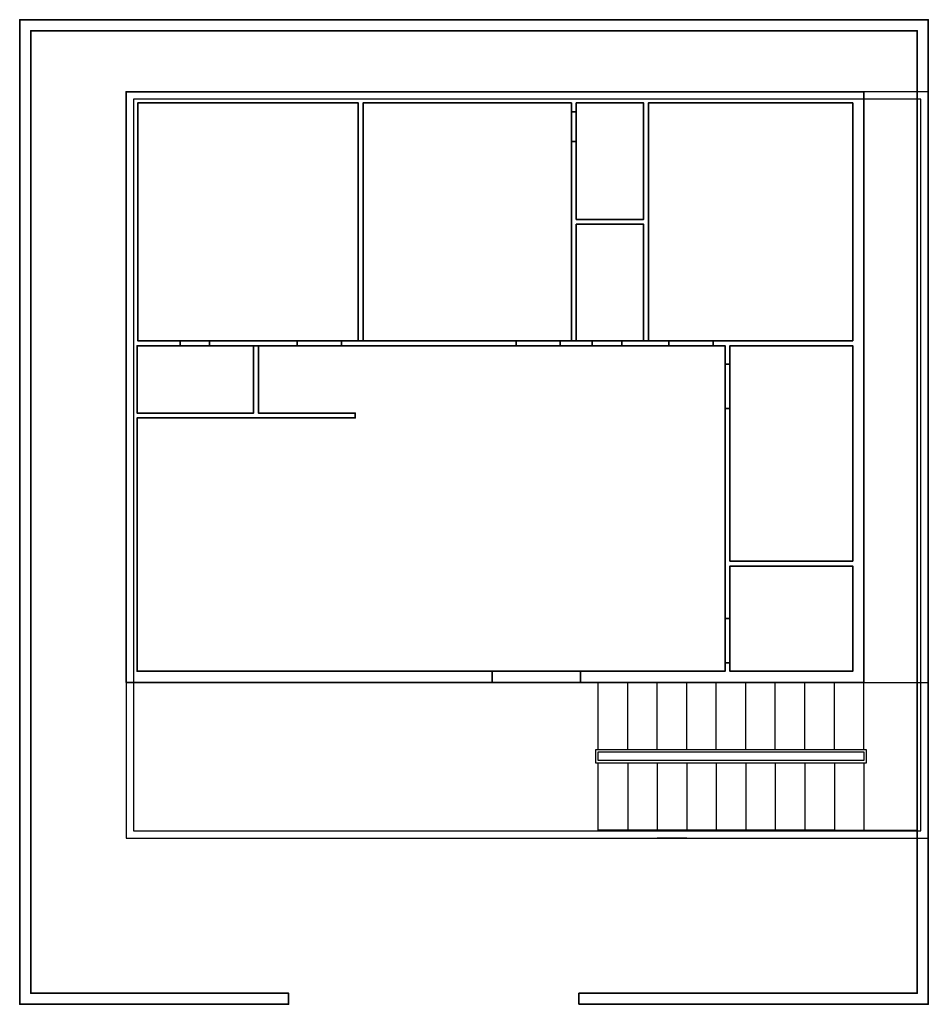
# Model space of a CAD drawing. Units: feet. Extents: x 3511 to 6270, y 2172 to 4127.
# Tile 3 of 4: x 5531 to 6270, y 2172 to 2972. Entities that reach past the tile are written whole.
import ezdxf

# ---------------------------------------------------------------- set-up
doc = ezdxf.new("R2010")
doc.units = ezdxf.units.FT
for name, color, linetype, lineweight in [('A-FLOR-OTLN', 3, 'Continuous', 25), ('A-FLOR-STRS', 4, 'Continuous', 25), ('A-WALL', 7, 'Continuous', 35), ('C-PROP', 1, 'Continuous', 35)]:
    doc.layers.add(name, color=color, linetype=linetype, lineweight=lineweight)

msp = doc.modelspace()

# ---------------------------------------------------------------- linework, layer by layer
at = {"layer": 'A-FLOR-OTLN', "elevation": 414}
for points in [[(5617.51, 2306.9), (6269.92, 2306.9), (6269.92, 2913.43), (5617.51, 2913.43)], [(5623.51, 2312.9), (6263.92, 2312.9), (6263.92, 2907.43), (5623.51, 2907.43)]]:
    msp.add_lwpolyline(points, close=True, dxfattribs=at)
at = {"layer": 'A-FLOR-STRS'}
for p, q in [((6001.51, 2379.01), (6001.51, 2433.43)), ((6025.51, 2379.01), (6025.51, 2433.43)), ((6049.51, 2379.01), (6049.51, 2433.43)), ((6073.51, 2379.01), (6073.51, 2433.43)), ((6097.51, 2379.01), (6097.51, 2433.43)), ((6121.51, 2379.01), (6121.51, 2433.43)), ((6145.51, 2379.01), (6145.51, 2433.43)), ((6169.51, 2379.01), (6169.51, 2433.43)), ((6193.51, 2379.01), (6193.51, 2433.43)), ((6260.92, 2433.43, 60), (6269.92, 2433.43, 60)), ((6269.92, 2306.9, 60), (6269.92, 2433.43, 60)), ((6217.51, 2367.86), (6217.51, 2313.43)), ((6217.51, 2313.43, 50.56), (6260.92, 2313.43, 50.56)), ((6049.51, 2306.9, 246), (6073.51, 2306.9, 246)), ((6073.51, 2306.9, 120), (6049.51, 2306.9, 120)), ((6260.92, 2306.9, 60), (6269.92, 2306.9, 60))]:
    msp.add_line(p, q, dxfattribs=at)
for points in [[(6217.51, 2379.01), (6217.51, 2433.43), (6260.92, 2433.43)], [(6025.51, 2367.86), (6025.51, 2313.43), (6013.51, 2313.43), (6001.51, 2313.43), (6001.51, 2367.86)], [(6049.51, 2367.86), (6049.51, 2313.43), (6037.51, 2313.43), (6025.51, 2313.43)], [(6073.51, 2367.86), (6073.51, 2313.43), (6061.51, 2313.43), (6049.51, 2313.43)], [(6097.51, 2367.86), (6097.51, 2313.43), (6085.51, 2313.43), (6073.51, 2313.43)], [(6121.51, 2367.86), (6121.51, 2313.43), (6109.51, 2313.43), (6097.51, 2313.43)], [(6145.51, 2367.86), (6145.51, 2313.43), (6133.51, 2313.43), (6121.51, 2313.43)], [(6169.51, 2367.86), (6169.51, 2313.43), (6157.51, 2313.43), (6145.51, 2313.43)], [(6193.51, 2367.86), (6193.51, 2313.43), (6181.51, 2313.43), (6169.51, 2313.43)], [(6193.51, 2313.43), (6205.51, 2313.43), (6217.51, 2313.43), (6260.92, 2313.43)]]:
    msp.add_lwpolyline(points, dxfattribs=at)
for points in [[(5999.51, 2379.01), (6219.51, 2379.01), (6219.51, 2367.86), (5999.51, 2367.86)], [(6217.51, 2369.86), (6001.51, 2369.86), (6001.51, 2377.01), (6217.51, 2377.01)]]:
    msp.add_lwpolyline(points, close=True, dxfattribs=at)
at = {"layer": 'A-WALL'}
msp.add_lwpolyline([(6108.6, 2528), (6108.6, 2485.38), (6104.6, 2485.38), (6104.6, 2656), (6108.6, 2656), (6108.6, 2532), (6208.51, 2532), (6208.51, 2707.06), (6108.6, 2707.06), (6108.6, 2692), (6104.6, 2692), (6104.6, 2707.06), (6094.92, 2707.06), (6094.92, 2711.06), (6208.51, 2711.06), (6208.51, 2904.43), (6042.38, 2904.43), (6042.38, 2711.06), (6058.92, 2711.06), (6058.92, 2707.06), (6020.61, 2707.06), (6020.61, 2711.06), (6038.38, 2711.06), (6038.38, 2805.75), (5983.67, 2805.75), (5983.67, 2711.06), (5996.61, 2711.06), (5996.61, 2707.06), (5970.67, 2707.06), (5970.67, 2711.06), (5979.67, 2711.06), (5979.67, 2873.18), (5983.67, 2873.18), (5983.67, 2809.75), (6038.38, 2809.75), (6038.38, 2904.43), (5983.67, 2904.43), (5983.67, 2897.18), (5979.67, 2897.18), (5979.67, 2904.43), (5810.34, 2904.43), (5810.34, 2711.06), (5934.67, 2711.06), (5934.67, 2707.06), (5792.78, 2707.06), (5792.78, 2711.06), (5806.34, 2711.06), (5806.34, 2904.43), (5627, 2904.43), (5627, 2711.06), (5661.53, 2711.06), (5661.53, 2707.06), (5626.51, 2707.06), (5626.51, 2652.36), (5626.51, 2652.36), (5721.2, 2652.36), (5721.2, 2707.07), (5685.53, 2707.07), (5685.53, 2711.07), (5756.78, 2711.07), (5756.78, 2707.07), (5725.2, 2707.07), (5725.2, 2652.36), (5803.95, 2652.36), (5803.95, 2648.36), (5626.51, 2648.36), (5626.51, 2442.43), (5915.15, 2442.43), (5915.15, 2433.43), (5617.51, 2433.43), (5617.51, 2913.43), (6217.51, 2913.43), (6217.51, 2433.43), (5987.15, 2433.43), (5987.15, 2442.43), (6104.6, 2442.43), (6104.6, 2449.38), (6108.6, 2449.38), (6108.6, 2442.43), (6208.51, 2442.43), (6208.51, 2528)], close=True, dxfattribs=at)
at = {"layer": 'A-WALL', "elevation": 120}
for points in [[(6217.51, 2433.43), (5617.51, 2433.43), (5617.51, 2913.43), (6217.51, 2913.43), (6217.51, 2433.43)], [(5806.34, 2711.06), (5806.34, 2904.43), (5627, 2904.43), (5627, 2711.06), (6208.51, 2711.06), (6208.51, 2904.43), (6042.38, 2904.43), (6042.38, 2711.06)], [(5979.67, 2904.43), (5810.34, 2904.43), (5810.34, 2711.06)], [(5979.67, 2711.06), (5979.67, 2904.43)], [(5983.67, 2904.43), (5983.67, 2809.75), (6038.38, 2809.75), (6038.38, 2904.43), (5983.67, 2904.43)], [(6038.38, 2711.06), (6038.38, 2805.75), (5983.67, 2805.75), (5983.67, 2711.06)], [(5725.2, 2707.07), (5725.2, 2652.36), (5803.95, 2652.36), (5803.95, 2648.36), (5626.51, 2648.36), (5626.51, 2442.43), (6104.6, 2442.43), (6104.6, 2707.06), (5626.51, 2707.06), (5626.51, 2652.36), (5626.51, 2652.36), (5721.2, 2652.36), (5721.2, 2707.07)], [(6108.6, 2707.06), (6108.6, 2532), (6208.51, 2532), (6208.51, 2707.06), (6108.6, 2707.06)], [(6108.6, 2442.43), (6208.51, 2442.43), (6208.51, 2528), (6108.6, 2528), (6108.6, 2442.43)]]:
    msp.add_lwpolyline(points, dxfattribs=at)
at = {"layer": 'A-WALL'}
msp.add_lwpolyline([(5725.2, 2648.36), (5725.2, 2648.36)], dxfattribs=at)
at = {"layer": 'C-PROP'}
msp.add_lwpolyline([(5985.75, 2171.8), (6269.92, 2171.8), (6269.92, 2972.04), (5531.06, 2972.04), (5531.06, 2171.8), (5749.68, 2171.8), (5749.68, 2180.8), (5540.06, 2180.8), (5540.06, 2963.04), (6260.92, 2963.04), (6260.92, 2180.8), (5985.75, 2180.8)], close=True, dxfattribs=at)

doc.saveas('drawing.dxf')
